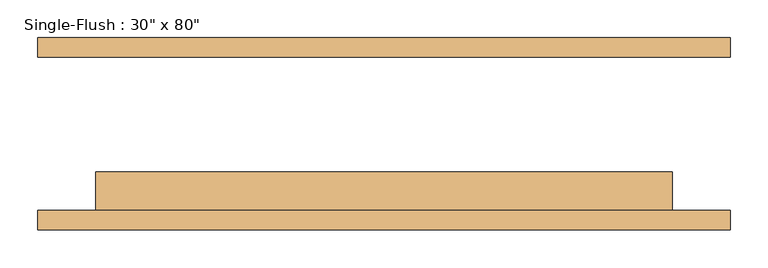
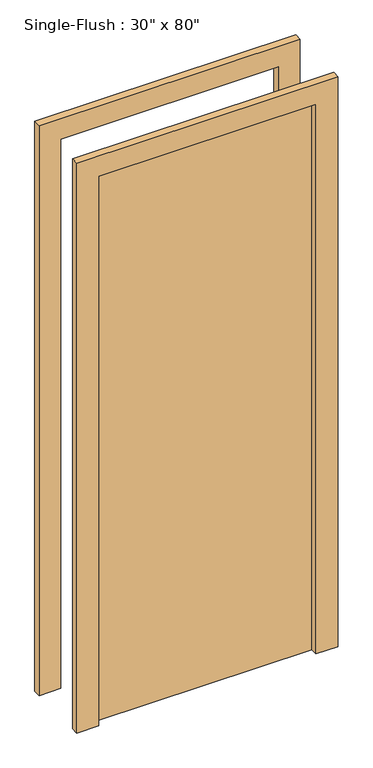
"""IFC4 building model written with IfcOpenShell, lengths in millimetres: door geometry."""

from ifc_helpers import new_model, si_unit, frame, origin, origin_with_axes, place, context, project, spatial, polyline, outline, extrude, source, transform, mapped, element, save


def door_53b1b562(model_context):
    return source(origin(), model_context, "Body", "SweptSolid", [
        extrude(outline(polyline([(2108.2, -457.2), (0.0, -457.2), (0.0, -381.0), (2032.0, -381.0), (2032.0, 381.0), (0.0, 381.0), (0.0, 457.2), (2108.2, 457.2), (2108.2, -457.2)])), frame((0.0, -127.0, 0.0), z_axis=(0.0, 1.0, 0.0), x_axis=(0.0, 0.0, 1.0)), (0.0, 0.0, 1.0), 25.4),
        extrude(outline(polyline([(2108.2, 457.2), (2108.2, -457.2), (0.0, -457.2), (0.0, -381.0), (2032.0, -381.0), (2032.0, 381.0), (0.0, 381.0), (0.0, 457.2), (2108.2, 457.2)])), frame((0.0, 101.6, 0.0), z_axis=(0.0, 1.0, 0.0), x_axis=(0.0, 0.0, 1.0)), (0.0, 0.0, 1.0), 25.4),
        extrude(outline(polyline([(381.0, -50.8), (381.0, -101.6), (-381.0, -101.6), (-381.0, -50.8), (381.0, -50.8)])), origin_with_axes(), (0.0, 0.0, 1.0), 2032.0),
    ])


if __name__ == "__main__":
    model = new_model("IFC4")
    model_context = context("Model", 3, world=origin())
    ifc_project = project(units=[si_unit("LENGTHUNIT", "METRE", prefix="MILLI")], contexts=[model_context])
    site = spatial("IfcSite", under=ifc_project)
    building = spatial("IfcBuilding", under=site)
    placement = place(None, origin())
    door_shape = door_53b1b562(model_context)
    element("IfcDoor", 1, ObjectType="Single-Flush : 30\" x 80\"", at=placement, inside=building, context=model_context, shape_type="MappedRepresentation", body=[
        mapped(door_shape, transform((0.0, 0.0, 0.0), x_axis=(1.0, 0.0, 0.0), y_axis=(0.0, 1.0, 0.0), z_axis=(0.0, 0.0, 1.0))),
    ])
    save(model, "model.ifc")

# Revit data of these elements
# Type "Single-Flush : 30\" x 80\""
#   Type Mark = "5"
#   Construction Type Id = "MDOOR"
#   Assembly Code = "C1020"
#   Analytic Construction = "Metal"
#   Thickness = 0' - 2"
#   Heat Transfer Coefficient (U) = 0.651978 BTU/(h·ft²·°F)
#   Height = 6' - 8"
#   Trim Projection Ext = 0' - 1"
#   Trim Projection Int = 0' - 1"
#   Trim Width = 0' - 3"
#   Width = 2' - 6"
#   Define Thermal Properties by = 1
#   Door Material = Door - Panel
#   Frame Material = Door - Frame
#   Visual Light Transmittance = 0
#   Solar Heat Gain Coefficient = 0
#   Function = (empty or 0)
#   Wall Closure = (empty or 0)
# Element 1 (IfcDoor, "Single-Flush : 30\" x 80\"")
#   Materials on its faces: "Door - Frame", "Door - Panel"
# Materials
#   "Door - Panel": class "Wood", colour RGB 210 159 95, transparency 0
#   "Door - Frame": colour RGB 118 70 51, transparency 0
